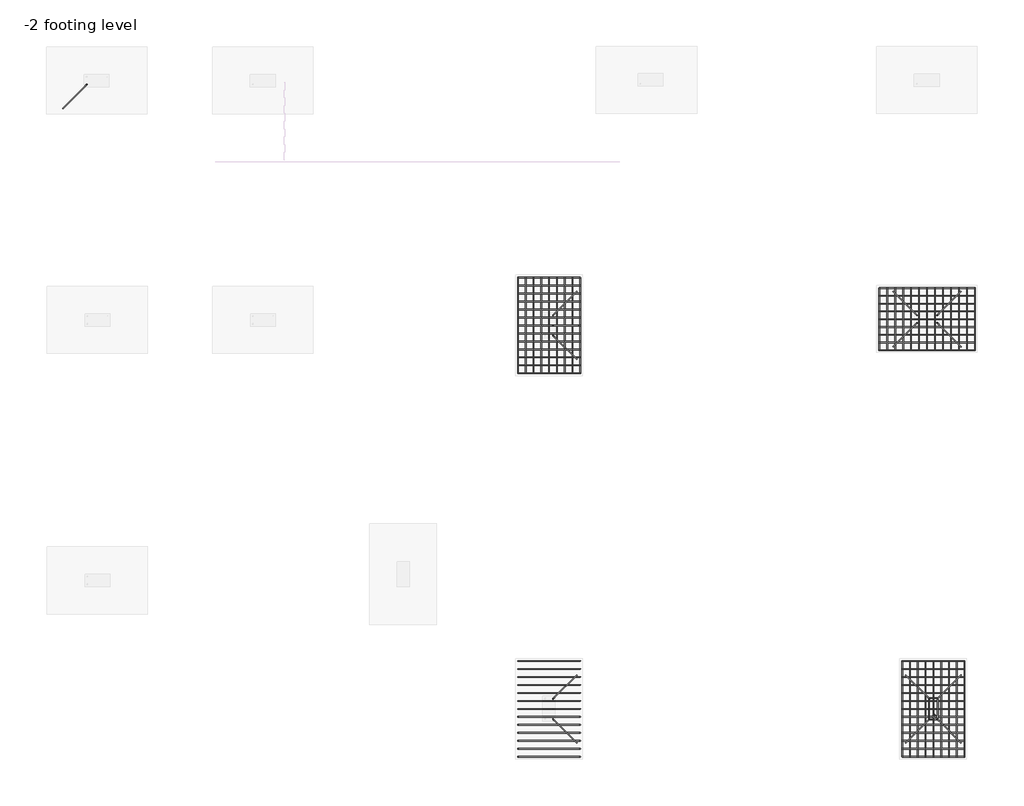
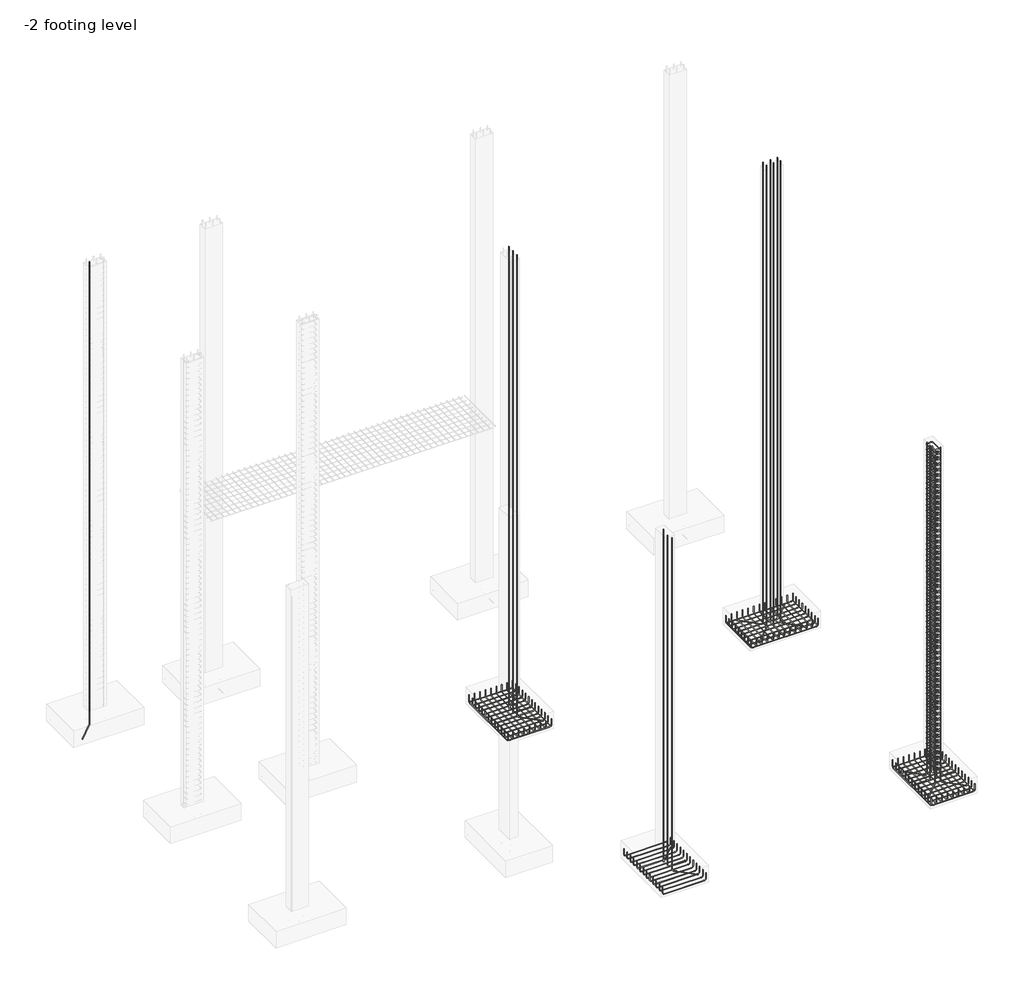
# One storey, part 4 of 9: 27 reinforcing bars.
"""IFC4 building model written with IfcOpenShell, lengths in millimetres."""

from ifc_helpers import new_model, si_unit, point, frame, origin, place, context, project, spatial, polyline, circle_curve, trimmed, segment, composite_curve, source, transform, mapped, element, save
from ifc_brep_helpers import swept_disk

model = new_model("IFC4")

# Units and contexts
model_context = context("Model", 3, world=origin())
ifc_project = project(units=[si_unit("LENGTHUNIT", "METRE", prefix="MILLI")], contexts=[model_context])

# Site, building, storey
site = spatial("IfcSite", under=ifc_project)
building = spatial("IfcBuilding", under=site)
storey = spatial("IfcBuildingStorey", under=building, Name="-2 footing level", Elevation=-1828.8)

# Reinforcing bars
placement = place(None, origin())
reinforcing_bar_shape = source(origin(), model_context, "Body", "SolidModel", [
    swept_disk(composite_curve([segment(polyline([(809.1088295, -3493.2851307, -2044.7), (809.1088295, -3493.2851307, -2197.1)]), True, "CONTINUOUS"), segment(trimmed(circle_curve(frame((809.1088295, -3448.8351307, -2197.1), z_axis=(1.0, 0.0, 0.0), x_axis=(0.0, -44.45000000000027, 0.0)), 44.45), [point((809.1088295, -3493.2851307, -2197.1))], [point((809.1088295, -3448.8351307, -2241.55))], True, "CARTESIAN"), True, "CONTINUOUS"), segment(polyline([(809.1088295, -3448.8351307, -2241.55), (809.1088295, -1797.8351307, -2241.55)]), True, "CONTINUOUS"), segment(trimmed(circle_curve(frame((809.1088295, -1797.8351307, -2197.1), z_axis=(1.0, 0.0, 0.0), x_axis=(0.0, 0.0, -44.45000000000027)), 44.45), [point((809.1088295, -1797.8351307, -2241.55))], [point((809.1088295, -1753.3851307, -2197.1))], True, "CARTESIAN"), True, "CONTINUOUS"), segment(polyline([(809.1088295, -1753.3851307, -2197.1), (809.1088295, -1753.3851307, -2044.7)]), True, "CONTINUOUS")], self_intersect=False), 6.35),
])
element("IfcReinforcingBar", 1, at=placement, inside=storey, context=model_context, shape_type="MappedRepresentation", body=[
    mapped(reinforcing_bar_shape, transform((0.0, 0.0, 0.0), x_axis=(1.0, 0.0, 0.0), y_axis=(0.0, 1.0, 0.0), z_axis=(0.0, 0.0, 1.0))),
    mapped(reinforcing_bar_shape, transform((-141.2875, 0.0, 0.0), x_axis=(1.0, 0.0, 0.0), y_axis=(0.0, 1.0, 0.0), z_axis=(0.0, 0.0, 1.0))),
    mapped(reinforcing_bar_shape, transform((-282.575, 0.0, 0.0), x_axis=(1.0, 0.0, 0.0), y_axis=(0.0, 1.0, 0.0), z_axis=(0.0, 0.0, 1.0))),
    mapped(reinforcing_bar_shape, transform((-423.8625, 0.0, 0.0), x_axis=(1.0, 0.0, 0.0), y_axis=(0.0, 1.0, 0.0), z_axis=(0.0, 0.0, 1.0))),
    mapped(reinforcing_bar_shape, transform((-565.15, 0.0, 0.0), x_axis=(1.0, 0.0, 0.0), y_axis=(0.0, 1.0, 0.0), z_axis=(0.0, 0.0, 1.0))),
    mapped(reinforcing_bar_shape, transform((-706.4375, 0.0, 0.0), x_axis=(1.0, 0.0, 0.0), y_axis=(0.0, 1.0, 0.0), z_axis=(0.0, 0.0, 1.0))),
    mapped(reinforcing_bar_shape, transform((-847.725, 0.0, 0.0), x_axis=(1.0, 0.0, 0.0), y_axis=(0.0, 1.0, 0.0), z_axis=(0.0, 0.0, 1.0))),
    mapped(reinforcing_bar_shape, transform((-989.0125, 0.0, 0.0), x_axis=(1.0, 0.0, 0.0), y_axis=(0.0, 1.0, 0.0), z_axis=(0.0, 0.0, 1.0))),
    mapped(reinforcing_bar_shape, transform((-1130.3, 0.0, 0.0), x_axis=(1.0, 0.0, 0.0), y_axis=(0.0, 1.0, 0.0), z_axis=(0.0, 0.0, 1.0))),
])
reinforcing_bar_2_shape = source(origin(), model_context, "Body", "SolidModel", [
    swept_disk(composite_curve([segment(polyline([(809.1088295, -1753.3851307, -2033.4041416), (809.1088295, -1753.3851307, -2185.8041416)]), True, "CONTINUOUS"), segment(trimmed(circle_curve(frame((764.6588295, -1753.3851307, -2185.8041416), z_axis=(0.0, 1.0, 0.0), x_axis=(44.44999999999993, 0.0, 0.0)), 44.45), [point((809.1088295, -1753.3851307, -2185.8041416))], [point((764.6588295, -1753.3851307, -2230.2541416))], True, "CARTESIAN"), True, "CONTINUOUS"), segment(polyline([(764.6588295, -1753.3851307, -2230.2541416), (-276.7411705, -1753.3851307, -2230.2541416)]), True, "CONTINUOUS"), segment(trimmed(circle_curve(frame((-276.7411705, -1753.3851307, -2185.8041416), z_axis=(0.0, 1.0, 0.0), x_axis=(0.0, 0.0, -44.44999999999982)), 44.45), [point((-276.7411705, -1753.3851307, -2230.2541416))], [point((-321.1911705, -1753.3851307, -2185.8041416))], True, "CARTESIAN"), True, "CONTINUOUS"), segment(polyline([(-321.1911705, -1753.3851307, -2185.8041416), (-321.1911705, -1753.3851307, -2033.4041416)]), True, "CONTINUOUS")], self_intersect=False), 6.35),
])
element("IfcReinforcingBar", 2, at=placement, inside=storey, context=model_context, shape_type="MappedRepresentation", body=[
    mapped(reinforcing_bar_2_shape, transform((0.0, 0.0, 0.0), x_axis=(1.0, 0.0, 0.0), y_axis=(0.0, 1.0, 0.0), z_axis=(0.0, 0.0, 1.0))),
    mapped(reinforcing_bar_2_shape, transform((0.0, -144.9916667, 0.0), x_axis=(1.0, 0.0, 0.0), y_axis=(0.0, 1.0, 0.0), z_axis=(0.0, 0.0, 1.0))),
    mapped(reinforcing_bar_2_shape, transform((0.0, -289.9833333, 0.0), x_axis=(1.0, 0.0, 0.0), y_axis=(0.0, 1.0, 0.0), z_axis=(0.0, 0.0, 1.0))),
    mapped(reinforcing_bar_2_shape, transform((0.0, -434.975, 0.0), x_axis=(1.0, 0.0, 0.0), y_axis=(0.0, 1.0, 0.0), z_axis=(0.0, 0.0, 1.0))),
    mapped(reinforcing_bar_2_shape, transform((0.0, -579.9666667, 0.0), x_axis=(1.0, 0.0, 0.0), y_axis=(0.0, 1.0, 0.0), z_axis=(0.0, 0.0, 1.0))),
    mapped(reinforcing_bar_2_shape, transform((0.0, -724.9583333, 0.0), x_axis=(1.0, 0.0, 0.0), y_axis=(0.0, 1.0, 0.0), z_axis=(0.0, 0.0, 1.0))),
    mapped(reinforcing_bar_2_shape, transform((0.0, -869.95, 0.0), x_axis=(1.0, 0.0, 0.0), y_axis=(0.0, 1.0, 0.0), z_axis=(0.0, 0.0, 1.0))),
    mapped(reinforcing_bar_2_shape, transform((0.0, -1014.9416667, 0.0), x_axis=(1.0, 0.0, 0.0), y_axis=(0.0, 1.0, 0.0), z_axis=(0.0, 0.0, 1.0))),
    mapped(reinforcing_bar_2_shape, transform((0.0, -1159.9333333, 0.0), x_axis=(1.0, 0.0, 0.0), y_axis=(0.0, 1.0, 0.0), z_axis=(0.0, 0.0, 1.0))),
    mapped(reinforcing_bar_2_shape, transform((0.0, -1304.925, 0.0), x_axis=(1.0, 0.0, 0.0), y_axis=(0.0, 1.0, 0.0), z_axis=(0.0, 0.0, 1.0))),
    mapped(reinforcing_bar_2_shape, transform((0.0, -1449.9166667, 0.0), x_axis=(1.0, 0.0, 0.0), y_axis=(0.0, 1.0, 0.0), z_axis=(0.0, 0.0, 1.0))),
    mapped(reinforcing_bar_2_shape, transform((0.0, -1594.9083333, 0.0), x_axis=(1.0, 0.0, 0.0), y_axis=(0.0, 1.0, 0.0), z_axis=(0.0, 0.0, 1.0))),
    mapped(reinforcing_bar_2_shape, transform((0.0, -1739.9, 0.0), x_axis=(1.0, 0.0, 0.0), y_axis=(0.0, 1.0, 0.0), z_axis=(0.0, 0.0, 1.0))),
])
reinforcing_bar_3_shape = source(origin(), model_context, "Body", "SolidModel", [
    swept_disk(composite_curve([segment(polyline([(6239.6679176, -3074.1851307, -2044.7), (6239.6679176, -3074.1851307, -2197.1)]), True, "CONTINUOUS"), segment(trimmed(circle_curve(frame((6284.1179176, -3074.1851307, -2197.1), z_axis=(0.0, -1.0, 0.0), x_axis=(-44.44999999999982, 0.0, 0.0)), 44.45), [point((6239.6679176, -3074.1851307, -2197.1))], [point((6284.1179176, -3074.1851307, -2241.55))], True, "CARTESIAN"), True, "CONTINUOUS"), segment(polyline([(6284.1179176, -3074.1851307, -2241.55), (7935.1179176, -3074.1851307, -2241.55)]), True, "CONTINUOUS"), segment(trimmed(circle_curve(frame((7935.1179176, -3074.1851307, -2197.1), z_axis=(0.0, -1.0, 0.0), x_axis=(0.0, 0.0, -44.45000000000027)), 44.45), [point((7935.1179176, -3074.1851307, -2241.55))], [point((7979.5679176, -3074.1851307, -2197.1))], True, "CARTESIAN"), True, "CONTINUOUS"), segment(polyline([(7979.5679176, -3074.1851307, -2197.1), (7979.5679176, -3074.1851307, -2044.7)]), True, "CONTINUOUS")], self_intersect=False), 6.35),
])
element("IfcReinforcingBar", 3, at=placement, inside=storey, context=model_context, shape_type="MappedRepresentation", body=[
    mapped(reinforcing_bar_3_shape, transform((0.0, 0.0, 0.0), x_axis=(1.0, 0.0, 0.0), y_axis=(0.0, 1.0, 0.0), z_axis=(0.0, 0.0, 1.0))),
    mapped(reinforcing_bar_3_shape, transform((0.0, 141.2875, 0.0), x_axis=(1.0, 0.0, 0.0), y_axis=(0.0, 1.0, 0.0), z_axis=(0.0, 0.0, 1.0))),
    mapped(reinforcing_bar_3_shape, transform((0.0, 282.575, 0.0), x_axis=(1.0, 0.0, 0.0), y_axis=(0.0, 1.0, 0.0), z_axis=(0.0, 0.0, 1.0))),
    mapped(reinforcing_bar_3_shape, transform((0.0, 423.8625, 0.0), x_axis=(1.0, 0.0, 0.0), y_axis=(0.0, 1.0, 0.0), z_axis=(0.0, 0.0, 1.0))),
    mapped(reinforcing_bar_3_shape, transform((0.0, 565.15, 0.0), x_axis=(1.0, 0.0, 0.0), y_axis=(0.0, 1.0, 0.0), z_axis=(0.0, 0.0, 1.0))),
    mapped(reinforcing_bar_3_shape, transform((0.0, 706.4375, 0.0), x_axis=(1.0, 0.0, 0.0), y_axis=(0.0, 1.0, 0.0), z_axis=(0.0, 0.0, 1.0))),
    mapped(reinforcing_bar_3_shape, transform((0.0, 847.725, 0.0), x_axis=(1.0, 0.0, 0.0), y_axis=(0.0, 1.0, 0.0), z_axis=(0.0, 0.0, 1.0))),
    mapped(reinforcing_bar_3_shape, transform((0.0, 989.0125, 0.0), x_axis=(1.0, 0.0, 0.0), y_axis=(0.0, 1.0, 0.0), z_axis=(0.0, 0.0, 1.0))),
    mapped(reinforcing_bar_3_shape, transform((0.0, 1130.3, 0.0), x_axis=(1.0, 0.0, 0.0), y_axis=(0.0, 1.0, 0.0), z_axis=(0.0, 0.0, 1.0))),
])
reinforcing_bar_4_shape = source(origin(), model_context, "Body", "SolidModel", [
    swept_disk(composite_curve([segment(polyline([(7979.5679176, -3074.1851307, -2033.4041416), (7979.5679176, -3074.1851307, -2185.8041416)]), True, "CONTINUOUS"), segment(trimmed(circle_curve(frame((7979.5679176, -3029.7351307, -2185.8041416), z_axis=(1.0, 0.0, 0.0), x_axis=(0.0, -44.45000000000027, 0.0)), 44.45), [point((7979.5679176, -3074.1851307, -2185.8041416))], [point((7979.5679176, -3029.7351307, -2230.2541416))], True, "CARTESIAN"), True, "CONTINUOUS"), segment(polyline([(7979.5679176, -3029.7351307, -2230.2541416), (7979.5679176, -1988.3351307, -2230.2541416)]), True, "CONTINUOUS"), segment(trimmed(circle_curve(frame((7979.5679176, -1988.3351307, -2185.8041416), z_axis=(1.0, 0.0, 0.0), x_axis=(0.0, 0.0, -44.44999999999982)), 44.45), [point((7979.5679176, -1988.3351307, -2230.2541416))], [point((7979.5679176, -1943.8851307, -2185.8041416))], True, "CARTESIAN"), True, "CONTINUOUS"), segment(polyline([(7979.5679176, -1943.8851307, -2185.8041416), (7979.5679176, -1943.8851307, -2033.4041416)]), True, "CONTINUOUS")], self_intersect=False), 6.35),
])
element("IfcReinforcingBar", 4, at=placement, inside=storey, context=model_context, shape_type="MappedRepresentation", body=[
    mapped(reinforcing_bar_4_shape, transform((0.0, 0.0, 0.0), x_axis=(1.0, 0.0, 0.0), y_axis=(0.0, 1.0, 0.0), z_axis=(0.0, 0.0, 1.0))),
    mapped(reinforcing_bar_4_shape, transform((-144.9916667, 0.0, 0.0), x_axis=(1.0, 0.0, 0.0), y_axis=(0.0, 1.0, 0.0), z_axis=(0.0, 0.0, 1.0))),
    mapped(reinforcing_bar_4_shape, transform((-289.9833333, 0.0, 0.0), x_axis=(1.0, 0.0, 0.0), y_axis=(0.0, 1.0, 0.0), z_axis=(0.0, 0.0, 1.0))),
    mapped(reinforcing_bar_4_shape, transform((-434.975, 0.0, 0.0), x_axis=(1.0, 0.0, 0.0), y_axis=(0.0, 1.0, 0.0), z_axis=(0.0, 0.0, 1.0))),
    mapped(reinforcing_bar_4_shape, transform((-579.9666667, 0.0, 0.0), x_axis=(1.0, 0.0, 0.0), y_axis=(0.0, 1.0, 0.0), z_axis=(0.0, 0.0, 1.0))),
    mapped(reinforcing_bar_4_shape, transform((-724.9583333, 0.0, 0.0), x_axis=(1.0, 0.0, 0.0), y_axis=(0.0, 1.0, 0.0), z_axis=(0.0, 0.0, 1.0))),
    mapped(reinforcing_bar_4_shape, transform((-869.95, 0.0, 0.0), x_axis=(1.0, 0.0, 0.0), y_axis=(0.0, 1.0, 0.0), z_axis=(0.0, 0.0, 1.0))),
    mapped(reinforcing_bar_4_shape, transform((-1014.9416667, 0.0, 0.0), x_axis=(1.0, 0.0, 0.0), y_axis=(0.0, 1.0, 0.0), z_axis=(0.0, 0.0, 1.0))),
    mapped(reinforcing_bar_4_shape, transform((-1159.9333333, 0.0, 0.0), x_axis=(1.0, 0.0, 0.0), y_axis=(0.0, 1.0, 0.0), z_axis=(0.0, 0.0, 1.0))),
    mapped(reinforcing_bar_4_shape, transform((-1304.925, 0.0, 0.0), x_axis=(1.0, 0.0, 0.0), y_axis=(0.0, 1.0, 0.0), z_axis=(0.0, 0.0, 1.0))),
    mapped(reinforcing_bar_4_shape, transform((-1449.9166667, 0.0, 0.0), x_axis=(1.0, 0.0, 0.0), y_axis=(0.0, 1.0, 0.0), z_axis=(0.0, 0.0, 1.0))),
    mapped(reinforcing_bar_4_shape, transform((-1594.9083333, 0.0, 0.0), x_axis=(1.0, 0.0, 0.0), y_axis=(0.0, 1.0, 0.0), z_axis=(0.0, 0.0, 1.0))),
    mapped(reinforcing_bar_4_shape, transform((-1739.9, 0.0, 0.0), x_axis=(1.0, 0.0, 0.0), y_axis=(0.0, 1.0, 0.0), z_axis=(0.0, 0.0, 1.0))),
])
reinforcing_bar_5_shape = source(origin(), model_context, "Body", "SolidModel", [
    swept_disk(composite_curve([segment(polyline([(-321.1911705, -10461.5294723, -2033.4041416), (-321.1911705, -10461.5294723, -2185.8041416)]), True, "CONTINUOUS"), segment(trimmed(circle_curve(frame((-276.7411705, -10461.5294723, -2185.8041416), z_axis=(0.0, -1.0, 0.0), x_axis=(-44.44999999999999, 0.0, 0.0)), 44.45), [point((-321.1911705, -10461.5294723, -2185.8041416))], [point((-276.7411705, -10461.5294723, -2230.2541416))], True, "CARTESIAN"), True, "CONTINUOUS"), segment(polyline([(-276.7411705, -10461.5294723, -2230.2541416), (764.6588295, -10461.5294723, -2230.2541416)]), True, "CONTINUOUS"), segment(trimmed(circle_curve(frame((764.6588295, -10461.5294723, -2185.8041416), z_axis=(0.0, -1.0, 0.0), x_axis=(0.0, 0.0, -44.44999999999982)), 44.45), [point((764.6588295, -10461.5294723, -2230.2541416))], [point((809.1088295, -10461.5294723, -2185.8041416))], True, "CARTESIAN"), True, "CONTINUOUS"), segment(polyline([(809.1088295, -10461.5294723, -2185.8041416), (809.1088295, -10461.5294723, -2033.4041416)]), True, "CONTINUOUS")], self_intersect=False), 6.35),
])
element("IfcReinforcingBar", 5, at=placement, inside=storey, context=model_context, shape_type="MappedRepresentation", body=[
    mapped(reinforcing_bar_5_shape, transform((0.0, 0.0, 0.0), x_axis=(1.0, 0.0, 0.0), y_axis=(0.0, 1.0, 0.0), z_axis=(0.0, 0.0, 1.0))),
    mapped(reinforcing_bar_5_shape, transform((0.0, 144.9916667, 0.0), x_axis=(1.0, 0.0, 0.0), y_axis=(0.0, 1.0, 0.0), z_axis=(0.0, 0.0, 1.0))),
    mapped(reinforcing_bar_5_shape, transform((0.0, 289.9833333, 0.0), x_axis=(1.0, 0.0, 0.0), y_axis=(0.0, 1.0, 0.0), z_axis=(0.0, 0.0, 1.0))),
    mapped(reinforcing_bar_5_shape, transform((0.0, 434.975, 0.0), x_axis=(1.0, 0.0, 0.0), y_axis=(0.0, 1.0, 0.0), z_axis=(0.0, 0.0, 1.0))),
    mapped(reinforcing_bar_5_shape, transform((0.0, 579.9666667, 0.0), x_axis=(1.0, 0.0, 0.0), y_axis=(0.0, 1.0, 0.0), z_axis=(0.0, 0.0, 1.0))),
    mapped(reinforcing_bar_5_shape, transform((0.0, 724.9583333, 0.0), x_axis=(1.0, 0.0, 0.0), y_axis=(0.0, 1.0, 0.0), z_axis=(0.0, 0.0, 1.0))),
    mapped(reinforcing_bar_5_shape, transform((0.0, 869.95, 0.0), x_axis=(1.0, 0.0, 0.0), y_axis=(0.0, 1.0, 0.0), z_axis=(0.0, 0.0, 1.0))),
    mapped(reinforcing_bar_5_shape, transform((0.0, 1014.9416667, 0.0), x_axis=(1.0, 0.0, 0.0), y_axis=(0.0, 1.0, 0.0), z_axis=(0.0, 0.0, 1.0))),
    mapped(reinforcing_bar_5_shape, transform((0.0, 1159.9333333, 0.0), x_axis=(1.0, 0.0, 0.0), y_axis=(0.0, 1.0, 0.0), z_axis=(0.0, 0.0, 1.0))),
    mapped(reinforcing_bar_5_shape, transform((0.0, 1304.925, 0.0), x_axis=(1.0, 0.0, 0.0), y_axis=(0.0, 1.0, 0.0), z_axis=(0.0, 0.0, 1.0))),
    mapped(reinforcing_bar_5_shape, transform((0.0, 1449.9166667, 0.0), x_axis=(1.0, 0.0, 0.0), y_axis=(0.0, 1.0, 0.0), z_axis=(0.0, 0.0, 1.0))),
    mapped(reinforcing_bar_5_shape, transform((0.0, 1594.9083333, 0.0), x_axis=(1.0, 0.0, 0.0), y_axis=(0.0, 1.0, 0.0), z_axis=(0.0, 0.0, 1.0))),
    mapped(reinforcing_bar_5_shape, transform((0.0, 1739.9, 0.0), x_axis=(1.0, 0.0, 0.0), y_axis=(0.0, 1.0, 0.0), z_axis=(0.0, 0.0, 1.0))),
])
reinforcing_bar_6_shape = source(origin(), model_context, "Body", "SolidModel", [
    swept_disk(composite_curve([segment(polyline([(6658.7679176, -8721.6294723, -2044.7), (6658.7679176, -8721.6294723, -2197.1)]), True, "CONTINUOUS"), segment(trimmed(circle_curve(frame((6658.7679176, -8766.0794723, -2197.1), z_axis=(-1.0, 0.0, 0.0), x_axis=(0.0, 44.45000000000073, 0.0)), 44.45), [point((6658.7679176, -8721.6294723, -2197.1))], [point((6658.7679176, -8766.0794723, -2241.55))], True, "CARTESIAN"), True, "CONTINUOUS"), segment(polyline([(6658.7679176, -8766.0794723, -2241.55), (6658.7679176, -10417.0794723, -2241.55)]), True, "CONTINUOUS"), segment(trimmed(circle_curve(frame((6658.7679176, -10417.0794723, -2197.1), z_axis=(-1.0, 0.0, 0.0), x_axis=(0.0, 0.0, -44.45000000000027)), 44.45), [point((6658.7679176, -10417.0794723, -2241.55))], [point((6658.7679176, -10461.5294723, -2197.1))], True, "CARTESIAN"), True, "CONTINUOUS"), segment(polyline([(6658.7679176, -10461.5294723, -2197.1), (6658.7679176, -10461.5294723, -2044.7)]), True, "CONTINUOUS")], self_intersect=False), 6.35),
])
element("IfcReinforcingBar", 6, at=placement, inside=storey, context=model_context, shape_type="MappedRepresentation", body=[
    mapped(reinforcing_bar_6_shape, transform((0.0, 0.0, 0.0), x_axis=(1.0, 0.0, 0.0), y_axis=(0.0, 1.0, 0.0), z_axis=(0.0, 0.0, 1.0))),
    mapped(reinforcing_bar_6_shape, transform((141.2875, 0.0, 0.0), x_axis=(1.0, 0.0, 0.0), y_axis=(0.0, 1.0, 0.0), z_axis=(0.0, 0.0, 1.0))),
    mapped(reinforcing_bar_6_shape, transform((282.575, 0.0, 0.0), x_axis=(1.0, 0.0, 0.0), y_axis=(0.0, 1.0, 0.0), z_axis=(0.0, 0.0, 1.0))),
    mapped(reinforcing_bar_6_shape, transform((423.8625, 0.0, 0.0), x_axis=(1.0, 0.0, 0.0), y_axis=(0.0, 1.0, 0.0), z_axis=(0.0, 0.0, 1.0))),
    mapped(reinforcing_bar_6_shape, transform((565.15, 0.0, 0.0), x_axis=(1.0, 0.0, 0.0), y_axis=(0.0, 1.0, 0.0), z_axis=(0.0, 0.0, 1.0))),
    mapped(reinforcing_bar_6_shape, transform((706.4375, 0.0, 0.0), x_axis=(1.0, 0.0, 0.0), y_axis=(0.0, 1.0, 0.0), z_axis=(0.0, 0.0, 1.0))),
    mapped(reinforcing_bar_6_shape, transform((847.725, 0.0, 0.0), x_axis=(1.0, 0.0, 0.0), y_axis=(0.0, 1.0, 0.0), z_axis=(0.0, 0.0, 1.0))),
    mapped(reinforcing_bar_6_shape, transform((989.0125, 0.0, 0.0), x_axis=(1.0, 0.0, 0.0), y_axis=(0.0, 1.0, 0.0), z_axis=(0.0, 0.0, 1.0))),
    mapped(reinforcing_bar_6_shape, transform((1130.3, 0.0, 0.0), x_axis=(1.0, 0.0, 0.0), y_axis=(0.0, 1.0, 0.0), z_axis=(0.0, 0.0, 1.0))),
])
reinforcing_bar_7_shape = source(origin(), model_context, "Body", "SolidModel", [
    swept_disk(composite_curve([segment(polyline([(6658.7679176, -10461.5294723, -2033.4041416), (6658.7679176, -10461.5294723, -2185.8041416)]), True, "CONTINUOUS"), segment(trimmed(circle_curve(frame((6703.2179176, -10461.5294723, -2185.8041416), z_axis=(0.0, -1.0, 0.0), x_axis=(-44.44999999999982, 0.0, 0.0)), 44.45), [point((6658.7679176, -10461.5294723, -2185.8041416))], [point((6703.2179176, -10461.5294723, -2230.2541416))], True, "CARTESIAN"), True, "CONTINUOUS"), segment(polyline([(6703.2179176, -10461.5294723, -2230.2541416), (7744.6179176, -10461.5294723, -2230.2541416)]), True, "CONTINUOUS"), segment(trimmed(circle_curve(frame((7744.6179176, -10461.5294723, -2185.8041416), z_axis=(0.0, -1.0, 0.0), x_axis=(0.0, 0.0, -44.44999999999982)), 44.45), [point((7744.6179176, -10461.5294723, -2230.2541416))], [point((7789.0679176, -10461.5294723, -2185.8041416))], True, "CARTESIAN"), True, "CONTINUOUS"), segment(polyline([(7789.0679176, -10461.5294723, -2185.8041416), (7789.0679176, -10461.5294723, -2033.4041416)]), True, "CONTINUOUS")], self_intersect=False), 6.35),
])
element("IfcReinforcingBar", 7, at=placement, inside=storey, context=model_context, shape_type="MappedRepresentation", body=[
    mapped(reinforcing_bar_7_shape, transform((0.0, 0.0, 0.0), x_axis=(1.0, 0.0, 0.0), y_axis=(0.0, 1.0, 0.0), z_axis=(0.0, 0.0, 1.0))),
    mapped(reinforcing_bar_7_shape, transform((0.0, 144.9916667, 0.0), x_axis=(1.0, 0.0, 0.0), y_axis=(0.0, 1.0, 0.0), z_axis=(0.0, 0.0, 1.0))),
    mapped(reinforcing_bar_7_shape, transform((0.0, 289.9833333, 0.0), x_axis=(1.0, 0.0, 0.0), y_axis=(0.0, 1.0, 0.0), z_axis=(0.0, 0.0, 1.0))),
    mapped(reinforcing_bar_7_shape, transform((0.0, 434.975, 0.0), x_axis=(1.0, 0.0, 0.0), y_axis=(0.0, 1.0, 0.0), z_axis=(0.0, 0.0, 1.0))),
    mapped(reinforcing_bar_7_shape, transform((0.0, 579.9666667, 0.0), x_axis=(1.0, 0.0, 0.0), y_axis=(0.0, 1.0, 0.0), z_axis=(0.0, 0.0, 1.0))),
    mapped(reinforcing_bar_7_shape, transform((0.0, 724.9583333, 0.0), x_axis=(1.0, 0.0, 0.0), y_axis=(0.0, 1.0, 0.0), z_axis=(0.0, 0.0, 1.0))),
    mapped(reinforcing_bar_7_shape, transform((0.0, 869.95, 0.0), x_axis=(1.0, 0.0, 0.0), y_axis=(0.0, 1.0, 0.0), z_axis=(0.0, 0.0, 1.0))),
    mapped(reinforcing_bar_7_shape, transform((0.0, 1014.9416667, 0.0), x_axis=(1.0, 0.0, 0.0), y_axis=(0.0, 1.0, 0.0), z_axis=(0.0, 0.0, 1.0))),
    mapped(reinforcing_bar_7_shape, transform((0.0, 1159.9333333, 0.0), x_axis=(1.0, 0.0, 0.0), y_axis=(0.0, 1.0, 0.0), z_axis=(0.0, 0.0, 1.0))),
    mapped(reinforcing_bar_7_shape, transform((0.0, 1304.925, 0.0), x_axis=(1.0, 0.0, 0.0), y_axis=(0.0, 1.0, 0.0), z_axis=(0.0, 0.0, 1.0))),
    mapped(reinforcing_bar_7_shape, transform((0.0, 1449.9166667, 0.0), x_axis=(1.0, 0.0, 0.0), y_axis=(0.0, 1.0, 0.0), z_axis=(0.0, 0.0, 1.0))),
    mapped(reinforcing_bar_7_shape, transform((0.0, 1594.9083333, 0.0), x_axis=(1.0, 0.0, 0.0), y_axis=(0.0, 1.0, 0.0), z_axis=(0.0, 0.0, 1.0))),
    mapped(reinforcing_bar_7_shape, transform((0.0, 1739.9, 0.0), x_axis=(1.0, 0.0, 0.0), y_axis=(0.0, 1.0, 0.0), z_axis=(0.0, 0.0, 1.0))),
])
element("IfcReinforcingBar", 8, at=placement, inside=storey, context=model_context, shape_type="SolidModel", body=[
    swept_disk(composite_curve([segment(polyline([(747.2623137, -3240.9386149, -2212.9582082), (345.2397259, -2838.9160271, -2212.9582082)]), True, "CONTINUOUS"), segment(trimmed(circle_curve(frame((345.2397259, -2838.9160271, -2168.5082082), z_axis=(0.7071067811865535, 0.7071067811865416, 0.0), x_axis=(0.0, 0.0, -44.45000000000027)), 44.45), [point((345.2397259, -2838.9160271, -2212.9582082))], [point((313.8088295, -2807.4851307, -2168.5082082))], True, "CARTESIAN"), True, "CONTINUOUS"), segment(polyline([(313.8088295, -2807.4851307, -2168.5082082), (313.8088295, -2807.4851307, 10477.5)]), True, "CONTINUOUS")], self_intersect=False), 6.35),
])
element("IfcReinforcingBar", 9, at=placement, inside=storey, context=model_context, shape_type="SolidModel", body=[
    swept_disk(composite_curve([segment(polyline([(747.2623137, -2005.7316465, -2212.9582082), (345.2397259, -2407.7542342, -2212.9582082)]), True, "CONTINUOUS"), segment(trimmed(circle_curve(frame((345.2397259, -2407.7542342, -2168.5082082), z_axis=(-0.7071067811865535, 0.7071067811865416, 0.0), x_axis=(0.0, 0.0, -44.45000000000027)), 44.45), [point((345.2397259, -2407.7542342, -2212.9582082))], [point((313.8088295, -2439.1851307, -2168.5082082))], True, "CARTESIAN"), True, "CONTINUOUS"), segment(polyline([(313.8088295, -2439.1851307, -2168.5082082), (313.8088295, -2439.1851307, 10477.5)]), True, "CONTINUOUS")], self_intersect=False), 6.35),
])
element("IfcReinforcingBar", 10, at=placement, inside=storey, context=model_context, shape_type="SolidModel", body=[
    swept_disk(composite_curve([segment(polyline([(771.0088295, -2623.3351307, -2212.9582082), (358.2588295, -2623.3351307, -2212.9582082)]), True, "CONTINUOUS"), segment(trimmed(circle_curve(frame((358.2588295, -2623.3351307, -2168.5082082), z_axis=(0.0, 1.0, 0.0), x_axis=(0.0, 0.0, -44.45000000000027)), 44.45), [point((358.2588295, -2623.3351307, -2212.9582082))], [point((313.8088295, -2623.3351307, -2168.5082082))], True, "CARTESIAN"), True, "CONTINUOUS"), segment(polyline([(313.8088295, -2623.3351307, -2168.5082082), (313.8088295, -2623.3351307, 10477.5)]), True, "CONTINUOUS")], self_intersect=False), 6.35),
])
element("IfcReinforcingBar", 11, at=placement, inside=storey, context=model_context, shape_type="SolidModel", body=[
    swept_disk(composite_curve([segment(polyline([(6720.012187, -10209.1829565, -2212.9582082), (7122.6370212, -9806.5581223, -2212.9582082)]), True, "CONTINUOUS"), segment(trimmed(circle_curve(frame((7122.6370212, -9806.5581223, -2168.5082082), z_axis=(0.7071067811865501, -0.7071067811865449, 0.0), x_axis=(0.0, 0.0, -44.45000000000027)), 44.45), [point((7122.6370212, -9806.5581223, -2212.9582082))], [point((7154.0679176, -9775.1272259, -2168.5082082))], True, "CARTESIAN"), True, "CONTINUOUS"), segment(polyline([(7154.0679176, -9775.1272259, -2168.5082082), (7154.0679176, -9775.1272259, 6778.6417918)]), True, "CONTINUOUS")], self_intersect=False), 6.35),
])
element("IfcReinforcingBar", 12, at=placement, inside=storey, context=model_context, shape_type="SolidModel", body=[
    swept_disk(composite_curve([segment(polyline([(7726.6191553, -10209.1829565, -2212.9582082), (7324.5965676, -9807.1603688, -2212.9582082)]), True, "CONTINUOUS"), segment(trimmed(circle_curve(frame((7324.5965676, -9807.1603688, -2168.5082082), z_axis=(0.7071067811865535, 0.7071067811865416, 0.0), x_axis=(0.0, 0.0, -44.45000000000027)), 44.45), [point((7324.5965676, -9807.1603688, -2212.9582082))], [point((7293.1656712, -9775.7294723, -2168.5082082))], True, "CARTESIAN"), True, "CONTINUOUS"), segment(polyline([(7293.1656712, -9775.7294723, -2168.5082082), (7293.1656712, -9775.7294723, 6972.3)]), True, "CONTINUOUS")], self_intersect=False), 6.35),
])
element("IfcReinforcingBar", 13, at=placement, inside=storey, context=model_context, shape_type="SolidModel", body=[
    swept_disk(composite_curve([segment(polyline([(6720.012187, -8973.9759881, -2212.9582082), (7122.6370212, -9376.6008224, -2212.9582082)]), True, "CONTINUOUS"), segment(trimmed(circle_curve(frame((7122.6370212, -9376.6008224, -2168.5082082), z_axis=(-0.7071067811865501, -0.7071067811865449, 0.0), x_axis=(0.0, 0.0, -44.45000000000027)), 44.45), [point((7122.6370212, -9376.6008224, -2212.9582082))], [point((7154.0679176, -9408.0317188, -2168.5082082))], True, "CARTESIAN"), True, "CONTINUOUS"), segment(polyline([(7154.0679176, -9408.0317188, -2168.5082082), (7154.0679176, -9408.0317188, 6931.0417918)]), True, "CONTINUOUS")], self_intersect=False), 6.35),
])
element("IfcReinforcingBar", 14, at=placement, inside=storey, context=model_context, shape_type="SolidModel", body=[
    swept_disk(composite_curve([segment(polyline([(7726.6191553, -8973.9759881, -2212.9582082), (7324.5965676, -9375.9985759, -2212.9582082)]), True, "CONTINUOUS"), segment(trimmed(circle_curve(frame((7324.5965676, -9375.9985759, -2168.5082082), z_axis=(-0.7071067811865535, 0.7071067811865416, 0.0), x_axis=(0.0, 0.0, -44.45000000000027)), 44.45), [point((7324.5965676, -9375.9985759, -2212.9582082))], [point((7293.1656712, -9407.4294723, -2168.5082082))], True, "CARTESIAN"), True, "CONTINUOUS"), segment(polyline([(7293.1656712, -9407.4294723, -2168.5082082), (7293.1656712, -9407.4294723, 6778.6417918)]), True, "CONTINUOUS")], self_intersect=False), 6.35),
])
element("IfcReinforcingBar", 15, at=placement, inside=storey, context=model_context, shape_type="SolidModel", body=[
    swept_disk(composite_curve([segment(polyline([(6696.2656712, -9591.5794723, -2212.9582082), (7080.1805388, -9591.5794723, -2212.9582082)]), True, "CONTINUOUS"), segment(trimmed(circle_curve(frame((7080.1805388, -9591.5794723, -2168.5082082), z_axis=(0.0, -1.0, 0.0), x_axis=(0.0, 0.0, -44.45000000000027)), 44.45), [point((7080.1805388, -9591.5794723, -2212.9582082))], [point((7124.6305388, -9591.5794723, -2168.5082082))], True, "CARTESIAN"), True, "CONTINUOUS"), segment(polyline([(7124.6305388, -9591.5794723, -2168.5082082), (7124.6305388, -9591.5794723, 6972.3)]), True, "CONTINUOUS")], self_intersect=False), 6.35),
])
element("IfcReinforcingBar", 16, at=placement, inside=storey, context=model_context, shape_type="SolidModel", body=[
    swept_disk(composite_curve([segment(polyline([(7750.3656712, -9591.5794723, -2212.9582082), (7336.2266087, -9591.5794723, -2212.9582082)]), True, "CONTINUOUS"), segment(trimmed(circle_curve(frame((7336.2266087, -9591.5794723, -2168.5082082), z_axis=(0.0, 1.0, 0.0), x_axis=(0.0, 0.0, -44.45000000000027)), 44.45), [point((7336.2266087, -9591.5794723, -2212.9582082))], [point((7291.7766087, -9591.5794723, -2168.5082082))], True, "CARTESIAN"), True, "CONTINUOUS"), segment(polyline([(7291.7766087, -9591.5794723, -2168.5082082), (7291.7766087, -9591.5794723, 6710.4417319)]), True, "CONTINUOUS")], self_intersect=False), 6.35),
])
reinforcing_bar_8_shape = source(origin(), model_context, "Body", "SolidModel", [
    swept_disk(composite_curve([segment(polyline([(7205.3744314, -9721.614193, -1794.0734375), (7262.2386284, -9778.4783901, -1794.0734375)]), True, "CONTINUOUS"), segment(trimmed(circle_curve(frame((7279.0766087, -9761.6404098, -1794.0734375), z_axis=(0.0, 0.0, 1.0), x_axis=(-16.8379802999998, -16.83798029999889, 0.0)), 23.8125), [point((7262.2386284, -9778.4783901, -1794.0734375))], [point((7302.8891087, -9761.6404098, -1794.0734375))], True, "CARTESIAN"), True, "CONTINUOUS"), segment(polyline([(7302.8891087, -9761.6404098, -1794.0734375), (7302.8891087, -9421.5185348, -1794.0734375)]), True, "CONTINUOUS"), segment(trimmed(circle_curve(frame((7279.0766087, -9421.5185348, -1794.0734375), z_axis=(0.0, 0.0, 1.0), x_axis=(23.8125, 0.0, 0.0)), 23.8125), [point((7302.8891087, -9421.5185348, -1794.0734375))], [point((7279.0766087, -9397.7060348, -1794.0734375))], True, "CARTESIAN"), True, "CONTINUOUS"), segment(polyline([(7279.0766087, -9397.7060348, -1794.0734375), (7167.5547337, -9397.7060348, -1794.0734375)]), True, "CONTINUOUS"), segment(trimmed(circle_curve(frame((7167.5547337, -9421.5113534, -1794.658215), z_axis=(0.0, -0.024557586497356516, 0.9996984169965585), x_axis=(0.0, 23.805318599999737, 0.5847774999999729)), 23.8125), [point((7167.5547337, -9397.7060348, -1794.0734375))], [point((7143.7422337, -9421.5113534, -1794.658215))], True, "CARTESIAN"), True, "CONTINUOUS"), segment(polyline([(7143.7422337, -9421.5113534, -1794.658215), (7143.7422337, -9761.6475913, -1803.01366)]), True, "CONTINUOUS"), segment(trimmed(circle_curve(frame((7167.5547337, -9761.6475913, -1803.01366), z_axis=(0.0, -0.024557586497356516, 0.9996984169965585), x_axis=(-23.8125, 0.0, 0.0)), 23.8125), [point((7143.7422337, -9761.6475913, -1803.01366))], [point((7167.5547337, -9785.4529098, -1803.5984375))], True, "CARTESIAN"), True, "CONTINUOUS"), segment(polyline([(7167.5547337, -9785.4529098, -1803.5984375), (7279.0766087, -9785.4529098, -1803.5984375)]), True, "CONTINUOUS"), segment(trimmed(circle_curve(frame((7279.0766087, -9761.6404098, -1803.5984375), z_axis=(0.0, 0.0, 1.0), x_axis=(0.0, -23.8125, 0.0)), 23.8125), [point((7279.0766087, -9785.4529098, -1803.5984375))], [point((7295.9145889, -9744.8024296, -1803.5984375))], True, "CARTESIAN"), True, "CONTINUOUS"), segment(polyline([(7295.9145889, -9744.8024296, -1803.5984375), (7239.0503918, -9687.9382325, -1803.5984375)]), True, "CONTINUOUS")], self_intersect=False), 4.7625),
])
element("IfcReinforcingBar", 17, at=placement, inside=storey, context=model_context, shape_type="MappedRepresentation", body=[
    mapped(reinforcing_bar_8_shape, transform((0.0, 0.0, 0.0), x_axis=(1.0, 0.0, 0.0), y_axis=(0.0, 1.0, 0.0), z_axis=(0.0, 0.0, 1.0))),
    mapped(reinforcing_bar_8_shape, transform((0.0, 0.0, 152.3249397), x_axis=(1.0, 0.0, 0.0), y_axis=(0.0, 1.0, 0.0), z_axis=(0.0, 0.0, 1.0))),
    mapped(reinforcing_bar_8_shape, transform((0.0, 0.0, 304.6498795), x_axis=(1.0, 0.0, 0.0), y_axis=(0.0, 1.0, 0.0), z_axis=(0.0, 0.0, 1.0))),
    mapped(reinforcing_bar_8_shape, transform((0.0, 0.0, 456.9748192), x_axis=(1.0, 0.0, 0.0), y_axis=(0.0, 1.0, 0.0), z_axis=(0.0, 0.0, 1.0))),
    mapped(reinforcing_bar_8_shape, transform((0.0, 0.0, 609.2997589), x_axis=(1.0, 0.0, 0.0), y_axis=(0.0, 1.0, 0.0), z_axis=(0.0, 0.0, 1.0))),
    mapped(reinforcing_bar_8_shape, transform((0.0, 0.0, 761.6246987), x_axis=(1.0, 0.0, 0.0), y_axis=(0.0, 1.0, 0.0), z_axis=(0.0, 0.0, 1.0))),
    mapped(reinforcing_bar_8_shape, transform((0.0, 0.0, 913.9496384), x_axis=(1.0, 0.0, 0.0), y_axis=(0.0, 1.0, 0.0), z_axis=(0.0, 0.0, 1.0))),
    mapped(reinforcing_bar_8_shape, transform((0.0, 0.0, 1066.2745781), x_axis=(1.0, 0.0, 0.0), y_axis=(0.0, 1.0, 0.0), z_axis=(0.0, 0.0, 1.0))),
    mapped(reinforcing_bar_8_shape, transform((0.0, 0.0, 1218.5995178), x_axis=(1.0, 0.0, 0.0), y_axis=(0.0, 1.0, 0.0), z_axis=(0.0, 0.0, 1.0))),
    mapped(reinforcing_bar_8_shape, transform((0.0, 0.0, 1370.9244576), x_axis=(1.0, 0.0, 0.0), y_axis=(0.0, 1.0, 0.0), z_axis=(0.0, 0.0, 1.0))),
    mapped(reinforcing_bar_8_shape, transform((0.0, 0.0, 1523.2493973), x_axis=(1.0, 0.0, 0.0), y_axis=(0.0, 1.0, 0.0), z_axis=(0.0, 0.0, 1.0))),
    mapped(reinforcing_bar_8_shape, transform((0.0, 0.0, 1675.574337), x_axis=(1.0, 0.0, 0.0), y_axis=(0.0, 1.0, 0.0), z_axis=(0.0, 0.0, 1.0))),
    mapped(reinforcing_bar_8_shape, transform((0.0, 0.0, 1827.8992768), x_axis=(1.0, 0.0, 0.0), y_axis=(0.0, 1.0, 0.0), z_axis=(0.0, 0.0, 1.0))),
    mapped(reinforcing_bar_8_shape, transform((0.0, 0.0, 1980.2242165), x_axis=(1.0, 0.0, 0.0), y_axis=(0.0, 1.0, 0.0), z_axis=(0.0, 0.0, 1.0))),
    mapped(reinforcing_bar_8_shape, transform((0.0, 0.0, 2132.5491562), x_axis=(1.0, 0.0, 0.0), y_axis=(0.0, 1.0, 0.0), z_axis=(0.0, 0.0, 1.0))),
    mapped(reinforcing_bar_8_shape, transform((0.0, 0.0, 2284.874096), x_axis=(1.0, 0.0, 0.0), y_axis=(0.0, 1.0, 0.0), z_axis=(0.0, 0.0, 1.0))),
    mapped(reinforcing_bar_8_shape, transform((0.0, 0.0, 2437.1990357), x_axis=(1.0, 0.0, 0.0), y_axis=(0.0, 1.0, 0.0), z_axis=(0.0, 0.0, 1.0))),
    mapped(reinforcing_bar_8_shape, transform((0.0, 0.0, 2589.5239754), x_axis=(1.0, 0.0, 0.0), y_axis=(0.0, 1.0, 0.0), z_axis=(0.0, 0.0, 1.0))),
    mapped(reinforcing_bar_8_shape, transform((0.0, 0.0, 2741.8489152), x_axis=(1.0, 0.0, 0.0), y_axis=(0.0, 1.0, 0.0), z_axis=(0.0, 0.0, 1.0))),
    mapped(reinforcing_bar_8_shape, transform((0.0, 0.0, 2894.1738549), x_axis=(1.0, 0.0, 0.0), y_axis=(0.0, 1.0, 0.0), z_axis=(0.0, 0.0, 1.0))),
    mapped(reinforcing_bar_8_shape, transform((0.0, 0.0, 3046.4987946), x_axis=(1.0, 0.0, 0.0), y_axis=(0.0, 1.0, 0.0), z_axis=(0.0, 0.0, 1.0))),
    mapped(reinforcing_bar_8_shape, transform((0.0, 0.0, 3198.8237343), x_axis=(1.0, 0.0, 0.0), y_axis=(0.0, 1.0, 0.0), z_axis=(0.0, 0.0, 1.0))),
    mapped(reinforcing_bar_8_shape, transform((0.0, 0.0, 3351.1486741), x_axis=(1.0, 0.0, 0.0), y_axis=(0.0, 1.0, 0.0), z_axis=(0.0, 0.0, 1.0))),
    mapped(reinforcing_bar_8_shape, transform((0.0, 0.0, 3503.4736138), x_axis=(1.0, 0.0, 0.0), y_axis=(0.0, 1.0, 0.0), z_axis=(0.0, 0.0, 1.0))),
    mapped(reinforcing_bar_8_shape, transform((0.0, 0.0, 3655.7985535), x_axis=(1.0, 0.0, 0.0), y_axis=(0.0, 1.0, 0.0), z_axis=(0.0, 0.0, 1.0))),
    mapped(reinforcing_bar_8_shape, transform((0.0, 0.0, 3808.1234933), x_axis=(1.0, 0.0, 0.0), y_axis=(0.0, 1.0, 0.0), z_axis=(0.0, 0.0, 1.0))),
    mapped(reinforcing_bar_8_shape, transform((0.0, 0.0, 3960.448433), x_axis=(1.0, 0.0, 0.0), y_axis=(0.0, 1.0, 0.0), z_axis=(0.0, 0.0, 1.0))),
    mapped(reinforcing_bar_8_shape, transform((0.0, 0.0, 4112.7733727), x_axis=(1.0, 0.0, 0.0), y_axis=(0.0, 1.0, 0.0), z_axis=(0.0, 0.0, 1.0))),
    mapped(reinforcing_bar_8_shape, transform((0.0, 0.0, 4265.0983125), x_axis=(1.0, 0.0, 0.0), y_axis=(0.0, 1.0, 0.0), z_axis=(0.0, 0.0, 1.0))),
    mapped(reinforcing_bar_8_shape, transform((0.0, 0.0, 4417.4232522), x_axis=(1.0, 0.0, 0.0), y_axis=(0.0, 1.0, 0.0), z_axis=(0.0, 0.0, 1.0))),
    mapped(reinforcing_bar_8_shape, transform((0.0, 0.0, 4569.7481919), x_axis=(1.0, 0.0, 0.0), y_axis=(0.0, 1.0, 0.0), z_axis=(0.0, 0.0, 1.0))),
    mapped(reinforcing_bar_8_shape, transform((0.0, 0.0, 4722.0731317), x_axis=(1.0, 0.0, 0.0), y_axis=(0.0, 1.0, 0.0), z_axis=(0.0, 0.0, 1.0))),
    mapped(reinforcing_bar_8_shape, transform((0.0, 0.0, 4874.3980714), x_axis=(1.0, 0.0, 0.0), y_axis=(0.0, 1.0, 0.0), z_axis=(0.0, 0.0, 1.0))),
    mapped(reinforcing_bar_8_shape, transform((0.0, 0.0, 5026.7230111), x_axis=(1.0, 0.0, 0.0), y_axis=(0.0, 1.0, 0.0), z_axis=(0.0, 0.0, 1.0))),
    mapped(reinforcing_bar_8_shape, transform((0.0, 0.0, 5179.0479508), x_axis=(1.0, 0.0, 0.0), y_axis=(0.0, 1.0, 0.0), z_axis=(0.0, 0.0, 1.0))),
    mapped(reinforcing_bar_8_shape, transform((0.0, 0.0, 5331.3728906), x_axis=(1.0, 0.0, 0.0), y_axis=(0.0, 1.0, 0.0), z_axis=(0.0, 0.0, 1.0))),
    mapped(reinforcing_bar_8_shape, transform((0.0, 0.0, 5483.6978303), x_axis=(1.0, 0.0, 0.0), y_axis=(0.0, 1.0, 0.0), z_axis=(0.0, 0.0, 1.0))),
    mapped(reinforcing_bar_8_shape, transform((0.0, 0.0, 5636.02277), x_axis=(1.0, 0.0, 0.0), y_axis=(0.0, 1.0, 0.0), z_axis=(0.0, 0.0, 1.0))),
    mapped(reinforcing_bar_8_shape, transform((0.0, 0.0, 5788.3477098), x_axis=(1.0, 0.0, 0.0), y_axis=(0.0, 1.0, 0.0), z_axis=(0.0, 0.0, 1.0))),
    mapped(reinforcing_bar_8_shape, transform((0.0, 0.0, 5940.6726495), x_axis=(1.0, 0.0, 0.0), y_axis=(0.0, 1.0, 0.0), z_axis=(0.0, 0.0, 1.0))),
    mapped(reinforcing_bar_8_shape, transform((0.0, 0.0, 6092.9975892), x_axis=(1.0, 0.0, 0.0), y_axis=(0.0, 1.0, 0.0), z_axis=(0.0, 0.0, 1.0))),
    mapped(reinforcing_bar_8_shape, transform((0.0, 0.0, 6245.322529), x_axis=(1.0, 0.0, 0.0), y_axis=(0.0, 1.0, 0.0), z_axis=(0.0, 0.0, 1.0))),
    mapped(reinforcing_bar_8_shape, transform((0.0, 0.0, 6397.6474687), x_axis=(1.0, 0.0, 0.0), y_axis=(0.0, 1.0, 0.0), z_axis=(0.0, 0.0, 1.0))),
    mapped(reinforcing_bar_8_shape, transform((0.0, 0.0, 6549.9724084), x_axis=(1.0, 0.0, 0.0), y_axis=(0.0, 1.0, 0.0), z_axis=(0.0, 0.0, 1.0))),
    mapped(reinforcing_bar_8_shape, transform((0.0, 0.0, 6702.2973482), x_axis=(1.0, 0.0, 0.0), y_axis=(0.0, 1.0, 0.0), z_axis=(0.0, 0.0, 1.0))),
    mapped(reinforcing_bar_8_shape, transform((0.0, 0.0, 6854.6222879), x_axis=(1.0, 0.0, 0.0), y_axis=(0.0, 1.0, 0.0), z_axis=(0.0, 0.0, 1.0))),
    mapped(reinforcing_bar_8_shape, transform((0.0, 0.0, 7006.9472276), x_axis=(1.0, 0.0, 0.0), y_axis=(0.0, 1.0, 0.0), z_axis=(0.0, 0.0, 1.0))),
    mapped(reinforcing_bar_8_shape, transform((0.0, 0.0, 7159.2721674), x_axis=(1.0, 0.0, 0.0), y_axis=(0.0, 1.0, 0.0), z_axis=(0.0, 0.0, 1.0))),
    mapped(reinforcing_bar_8_shape, transform((0.0, 0.0, 7311.5971071), x_axis=(1.0, 0.0, 0.0), y_axis=(0.0, 1.0, 0.0), z_axis=(0.0, 0.0, 1.0))),
    mapped(reinforcing_bar_8_shape, transform((0.0, 0.0, 7463.9220468), x_axis=(1.0, 0.0, 0.0), y_axis=(0.0, 1.0, 0.0), z_axis=(0.0, 0.0, 1.0))),
    mapped(reinforcing_bar_8_shape, transform((0.0, 0.0, 7616.2469865), x_axis=(1.0, 0.0, 0.0), y_axis=(0.0, 1.0, 0.0), z_axis=(0.0, 0.0, 1.0))),
    mapped(reinforcing_bar_8_shape, transform((0.0, 0.0, 7768.5719263), x_axis=(1.0, 0.0, 0.0), y_axis=(0.0, 1.0, 0.0), z_axis=(0.0, 0.0, 1.0))),
    mapped(reinforcing_bar_8_shape, transform((0.0, 0.0, 7920.896866), x_axis=(1.0, 0.0, 0.0), y_axis=(0.0, 1.0, 0.0), z_axis=(0.0, 0.0, 1.0))),
    mapped(reinforcing_bar_8_shape, transform((0.0, 0.0, 8073.2218057), x_axis=(1.0, 0.0, 0.0), y_axis=(0.0, 1.0, 0.0), z_axis=(0.0, 0.0, 1.0))),
    mapped(reinforcing_bar_8_shape, transform((0.0, 0.0, 8225.5467455), x_axis=(1.0, 0.0, 0.0), y_axis=(0.0, 1.0, 0.0), z_axis=(0.0, 0.0, 1.0))),
    mapped(reinforcing_bar_8_shape, transform((0.0, 0.0, 8377.8716852), x_axis=(1.0, 0.0, 0.0), y_axis=(0.0, 1.0, 0.0), z_axis=(0.0, 0.0, 1.0))),
    mapped(reinforcing_bar_8_shape, transform((0.0, 0.0, 8530.1966249), x_axis=(1.0, 0.0, 0.0), y_axis=(0.0, 1.0, 0.0), z_axis=(0.0, 0.0, 1.0))),
    mapped(reinforcing_bar_8_shape, transform((0.0, 0.0, 8682.5215647), x_axis=(1.0, 0.0, 0.0), y_axis=(0.0, 1.0, 0.0), z_axis=(0.0, 0.0, 1.0))),
])
element("IfcReinforcingBar", 18, at=placement, inside=storey, context=model_context, shape_type="SolidModel", body=[
    swept_disk(composite_curve([segment(polyline([(747.2623137, -10209.1829565, -2212.9582082), (345.2397259, -9807.1603688, -2212.9582082)]), True, "CONTINUOUS"), segment(trimmed(circle_curve(frame((345.2397259, -9807.1603688, -2168.5082082), z_axis=(0.7071067811865535, 0.7071067811865416, 0.0), x_axis=(0.0, 0.0, -44.45000000000027)), 44.45), [point((345.2397259, -9807.1603688, -2212.9582082))], [point((313.8088295, -9775.7294723, -2168.5082082))], True, "CARTESIAN"), True, "CONTINUOUS"), segment(polyline([(313.8088295, -9775.7294723, -2168.5082082), (313.8088295, -9775.7294723, 6931.0417918)]), True, "CONTINUOUS")], self_intersect=False), 6.35),
])
element("IfcReinforcingBar", 19, at=placement, inside=storey, context=model_context, shape_type="SolidModel", body=[
    swept_disk(composite_curve([segment(polyline([(747.2623137, -8973.9759881, -2212.9582082), (345.2397259, -9375.9985759, -2212.9582082)]), True, "CONTINUOUS"), segment(trimmed(circle_curve(frame((345.2397259, -9375.9985759, -2168.5082082), z_axis=(-0.7071067811865535, 0.7071067811865416, 0.0), x_axis=(0.0, 0.0, -44.45000000000027)), 44.45), [point((345.2397259, -9375.9985759, -2212.9582082))], [point((313.8088295, -9407.4294723, -2168.5082082))], True, "CARTESIAN"), True, "CONTINUOUS"), segment(polyline([(313.8088295, -9407.4294723, -2168.5082082), (313.8088295, -9407.4294723, 6931.0417918)]), True, "CONTINUOUS")], self_intersect=False), 6.35),
])
element("IfcReinforcingBar", 20, at=placement, inside=storey, context=model_context, shape_type="SolidModel", body=[
    swept_disk(composite_curve([segment(polyline([(771.0088295, -9591.5794723, -2212.9582082), (356.869767, -9591.5794723, -2212.9582082)]), True, "CONTINUOUS"), segment(trimmed(circle_curve(frame((356.869767, -9591.5794723, -2168.5082082), z_axis=(0.0, 1.0, 0.0), x_axis=(0.0, 0.0, -44.45000000000027)), 44.45), [point((356.869767, -9591.5794723, -2212.9582082))], [point((312.419767, -9591.5794723, -2168.5082082))], True, "CARTESIAN"), True, "CONTINUOUS"), segment(polyline([(312.419767, -9591.5794723, -2168.5082082), (312.419767, -9591.5794723, 6881.3072244)]), True, "CONTINUOUS")], self_intersect=False), 6.35),
])
element("IfcReinforcingBar", 21, at=placement, inside=storey, context=model_context, shape_type="SolidModel", body=[
    swept_disk(composite_curve([segment(polyline([(6491.412187, -2003.8410883, -2212.9582082), (6893.4347747, -2405.8636761, -2212.9582082)]), True, "CONTINUOUS"), segment(trimmed(circle_curve(frame((6893.4347747, -2405.8636761, -2168.5082082), z_axis=(-0.7071067811865455, -0.7071067811865496, 0.0), x_axis=(0.0, 0.0, -44.45000000000027)), 44.45), [point((6893.4347747, -2405.8636761, -2212.9582082))], [point((6924.8656712, -2437.2945725, -2168.5082082))], True, "CARTESIAN"), True, "CONTINUOUS"), segment(polyline([(6924.8656712, -2437.2945725, -2168.5082082), (6924.8656712, -2437.2945725, 10477.5)]), True, "CONTINUOUS")], self_intersect=False), 6.35),
])
element("IfcReinforcingBar", 22, at=placement, inside=storey, context=model_context, shape_type="SolidModel", body=[
    swept_disk(composite_curve([segment(polyline([(6491.412187, -3010.4480567, -2212.9582082), (6893.4347747, -2608.4254689, -2212.9582082)]), True, "CONTINUOUS"), segment(trimmed(circle_curve(frame((6893.4347747, -2608.4254689, -2168.5082082), z_axis=(0.707106781186541, -0.707106781186554, 0.0), x_axis=(0.0, 0.0, -44.45000000000027)), 44.45), [point((6893.4347747, -2608.4254689, -2212.9582082))], [point((6924.8656712, -2576.9945725, -2168.5082082))], True, "CARTESIAN"), True, "CONTINUOUS"), segment(polyline([(6924.8656712, -2576.9945725, -2168.5082082), (6924.8656712, -2576.9945725, 10477.5)]), True, "CONTINUOUS")], self_intersect=False), 6.35),
])
element("IfcReinforcingBar", 23, at=placement, inside=storey, context=model_context, shape_type="SolidModel", body=[
    swept_disk(composite_curve([segment(polyline([(7726.6191553, -2003.8410883, -2212.9582082), (7324.5965676, -2405.8636761, -2212.9582082)]), True, "CONTINUOUS"), segment(trimmed(circle_curve(frame((7324.5965676, -2405.8636761, -2168.5082082), z_axis=(-0.7071067811865444, 0.7071067811865507, 0.0), x_axis=(0.0, 0.0, -44.45000000000027)), 44.45), [point((7324.5965676, -2405.8636761, -2212.9582082))], [point((7293.1656712, -2437.2945725, -2168.5082082))], True, "CARTESIAN"), True, "CONTINUOUS"), segment(polyline([(7293.1656712, -2437.2945725, -2168.5082082), (7293.1656712, -2437.2945725, 10477.5)]), True, "CONTINUOUS")], self_intersect=False), 6.35),
])
element("IfcReinforcingBar", 24, at=placement, inside=storey, context=model_context, shape_type="SolidModel", body=[
    swept_disk(composite_curve([segment(polyline([(7726.6191553, -3010.4480567, -2212.9582082), (7324.5965676, -2608.4254689, -2212.9582082)]), True, "CONTINUOUS"), segment(trimmed(circle_curve(frame((7324.5965676, -2608.4254689, -2168.5082082), z_axis=(0.7071067811865421, 0.7071067811865529, 0.0), x_axis=(0.0, 0.0, -44.45000000000027)), 44.45), [point((7324.5965676, -2608.4254689, -2212.9582082))], [point((7293.1656712, -2576.9945725, -2168.5082082))], True, "CARTESIAN"), True, "CONTINUOUS"), segment(polyline([(7293.1656712, -2576.9945725, -2168.5082082), (7293.1656712, -2576.9945725, 10477.5)]), True, "CONTINUOUS")], self_intersect=False), 6.35),
])
element("IfcReinforcingBar", 25, at=placement, inside=storey, context=model_context, shape_type="SolidModel", body=[
    swept_disk(composite_curve([segment(polyline([(7109.0156712, -1980.0945725, -2212.9582082), (7109.0156712, -2394.233635, -2212.9582082)]), True, "CONTINUOUS"), segment(trimmed(circle_curve(frame((7109.0156712, -2394.233635, -2168.5082082), z_axis=(-1.0, 0.0, 0.0), x_axis=(0.0, 0.0, -44.45000000000027)), 44.45), [point((7109.0156712, -2394.233635, -2212.9582082))], [point((7109.0156712, -2438.683635, -2168.5082082))], True, "CARTESIAN"), True, "CONTINUOUS"), segment(polyline([(7109.0156712, -2438.683635, -2168.5082082), (7109.0156712, -2438.683635, 10477.5)]), True, "CONTINUOUS")], self_intersect=False), 6.35),
])
element("IfcReinforcingBar", 26, at=placement, inside=storey, context=model_context, shape_type="SolidModel", body=[
    swept_disk(composite_curve([segment(polyline([(7109.0156712, -3034.1945725, -2212.9582082), (7109.0156712, -2620.05551, -2212.9582082)]), True, "CONTINUOUS"), segment(trimmed(circle_curve(frame((7109.0156712, -2620.05551, -2168.5082082), z_axis=(1.0, 0.0, 0.0), x_axis=(0.0, 0.0, -44.45000000000027)), 44.45), [point((7109.0156712, -2620.05551, -2212.9582082))], [point((7109.0156712, -2575.60551, -2168.5082082))], True, "CARTESIAN"), True, "CONTINUOUS"), segment(polyline([(7109.0156712, -2575.60551, -2168.5082082), (7109.0156712, -2575.60551, 10477.5)]), True, "CONTINUOUS")], self_intersect=False), 6.35),
])
element("IfcReinforcingBar", 27, at=placement, inside=storey, context=model_context, shape_type="SolidModel", body=[
    swept_disk(composite_curve([segment(polyline([(-8587.4414927, 1321.6659151, -2212.9582082), (-8185.4189049, 1723.6885028, -2212.9582082)]), True, "CONTINUOUS"), segment(trimmed(circle_curve(frame((-8185.4189049, 1723.6885028, -2168.5082082), z_axis=(0.707106781186541, -0.707106781186554, 0.0), x_axis=(0.0, 0.0, -44.45000000000027)), 44.45), [point((-8185.4189049, 1723.6885028, -2212.9582082))], [point((-8153.9880085, 1755.1193993, -2168.5082082))], True, "CARTESIAN"), True, "CONTINUOUS"), segment(polyline([(-8153.9880085, 1755.1193993, -2168.5082082), (-8153.9880085, 1755.1193993, 10477.5)]), True, "CONTINUOUS")], self_intersect=False), 6.35),
])

save(model, "model.ifc")

# Revit data of these elements
# Elements 1, 2, 3, 4, 5, 6, 7, 8, 9, 10, 11, 12, 13, 14, 15, 16, 17, 18, 19, 20, 21, 22, 23, 24, 25, 26, 27 (IfcReinforcingBar)
#   Phase Created = New Construction
